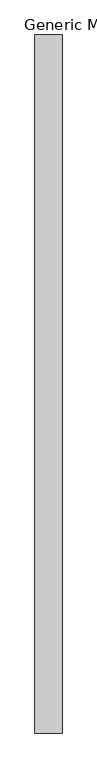
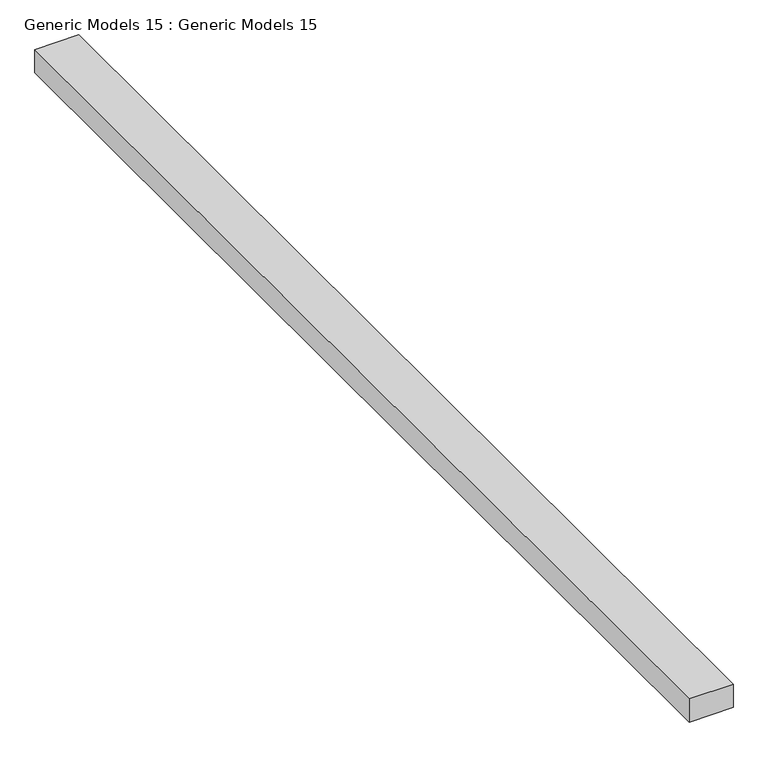
"""IFC4 building model written with IfcOpenShell, lengths in millimetres: proxy geometry, Generic Models 15 : Generic Models 15."""

from ifc_helpers import new_model, si_unit, frame, origin, place, context, project, spatial, polyline, outline, extrude, source, transform, mapped, element, save


def generic_models_15_generic_models_15_8aebc9bb(model_context):
    return source(origin(), model_context, "Body", "SweptSolid", [
        extrude(outline(polyline([(-15779.038419, -5947.7713044), (-15779.038419, 6968.9307139), (-15276.638074, 6968.9307139), (-15276.638074, -5947.7713044), (-15779.038419, -5947.7713044)])), frame((0.0, 0.0, 29629.1), z_axis=(0.0, 0.0, 1.0), x_axis=(1.0, 0.0, 0.0)), (0.0, 0.0, 1.0), 279.4561104),
    ])


if __name__ == "__main__":
    model = new_model("IFC4")
    model_context = context("Model", 3, world=origin())
    ifc_project = project(units=[si_unit("LENGTHUNIT", "METRE", prefix="MILLI")], contexts=[model_context])
    site = spatial("IfcSite", under=ifc_project)
    building = spatial("IfcBuilding", under=site)
    placement = place(None, origin())
    generic_models_15_generic_models_15_shape = generic_models_15_generic_models_15_8aebc9bb(model_context)
    element("IfcBuildingElementProxy", 1, Name="Generic Models 15 : Generic Models 15", ObjectType="Generic Models 15 : Generic Models 15", at=placement, inside=building, context=model_context, shape_type="MappedRepresentation", body=[
        mapped(generic_models_15_generic_models_15_shape, transform((0.0, 0.0, 0.0), x_axis=(1.0, 0.0, 0.0), y_axis=(0.0, 1.0, 0.0), z_axis=(0.0, 0.0, 1.0))),
    ])
    save(model, "model.ifc")
